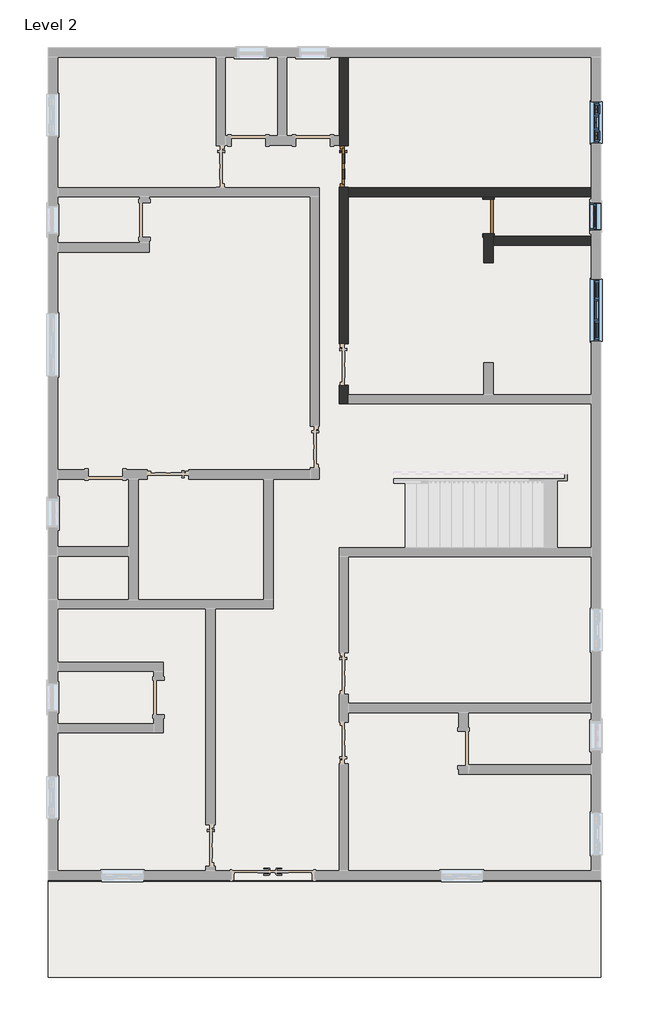
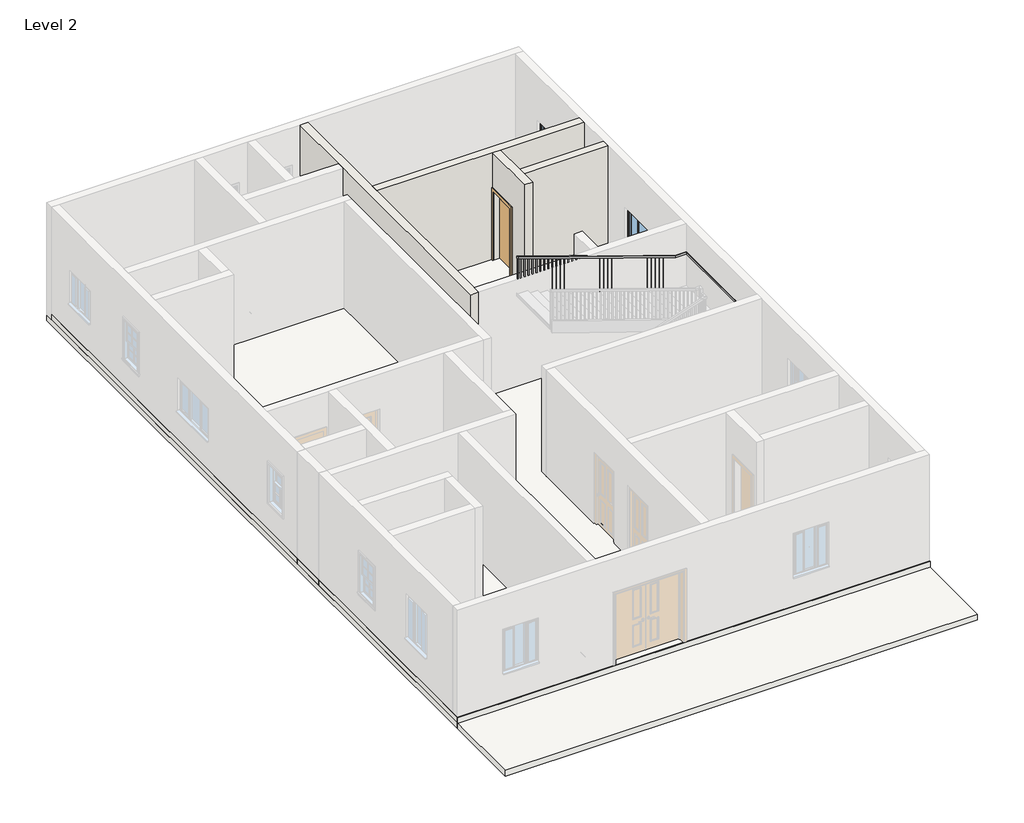
# One storey, part 2 of 3: 4 walls, 3 windows, 2 doors, 2 roofs, 2 slabs, 1 railing.
"""IFC4 building model written with IfcOpenShell, lengths in millimetres."""

from ifc_helpers import new_model, si_unit, frame, origin, place, context, project, spatial, polyline, outline, extrude, faceted_brep, transform, mapped, element, save
from components import door_51b0c682, door_fadea3f2, window_679d2811, windows_tpl_plain_1360x910mm_84993ef1, windows_tpl_w_glazing_cross_bars_910x910mm_4aa0f884

model = new_model("IFC4")

# Units and contexts
model_context = context("Model", 3, world=origin())
ifc_project = project(units=[si_unit("LENGTHUNIT", "METRE", prefix="MILLI")], contexts=[model_context])

# Site, building, storey
site = spatial("IfcSite", under=ifc_project)
building = spatial("IfcBuilding", under=site)
storey = spatial("IfcBuildingStorey", under=building, Name="Level 2", Elevation=3048.0)

# Doors
placement = place(None, origin())
door_shape = door_51b0c682(model_context)
element("IfcDoor", 1, ObjectType="Doors_ExtSgl_2 : 2'x7\"", at=placement, inside=storey, context=model_context, shape_type="MappedRepresentation", body=[
    mapped(door_shape, transform((348.5548051, 6357.8803322, 3048.0), x_axis=(0.0, -1.0, 0.0), y_axis=(1.0, 0.0, 0.0), z_axis=(0.0, 0.0, 1.0))),
])
door_2_shape = door_fadea3f2(model_context)
element("IfcDoor", 2, ObjectType="Single-Flush : 30\" x 80\"", at=placement, inside=storey, context=model_context, shape_type="MappedRepresentation", body=[
    mapped(door_2_shape, transform((3523.5548051, 5259.3303322, 3048.0), x_axis=(0.0, -1.0, 0.0), y_axis=(1.0, 0.0, 0.0), z_axis=(0.0, 0.0, 1.0))),
])

# Railing
element("IfcRailing", 3, ObjectType="Handrail - Rectangular", at=placement, inside=storey, context=model_context, shape_type="SolidModel", body=[
    faceted_brep([(1449.3932247, -2014.4659014, 4048.125), (1449.3932247, -2014.4659014, 3994.4913852), (1449.3932247, -2065.2659014, 3994.4913852), (1449.3932247, -2065.2659014, 4048.125), (5246.6669505, -2014.4659014, 5334.0), (5255.0348019, -2014.4659014, 5283.2), (5255.0348019, -2065.2659014, 5283.2), (5246.6669505, -2065.2659014, 5334.0), (5771.4548051, -2014.4659014, 5334.0), (5771.4548051, -2014.4659014, 5283.2), (5822.2548051, -2065.2659014, 5283.2), (5822.2548051, -2065.2659014, 5334.0), (5771.4548051, 1135.1340986, 5334.0), (5771.4548051, 1135.1340986, 5283.2), (5822.2548051, 1185.9340986, 5283.2), (5822.2548051, 1185.9340986, 5334.0), (5499.8185322, 1135.1340986, 5334.0), (5491.4506807, 1135.1340986, 5283.2), (5491.4506807, 1185.9340986, 5283.2), (5499.8185322, 1185.9340986, 5334.0), (1449.3932247, 1135.1340986, 6705.6), (1449.3932247, 1185.9340986, 6705.6), (1449.3932247, 1185.9340986, 6651.9663852), (1449.3932247, 1135.1340986, 6651.9663852)], [[[0, 1, 2, 3]], [[1, 0, 4, 5]], [[2, 1, 5, 6]], [[3, 2, 6, 7]], [[0, 3, 7, 4]], [[5, 4, 8, 9]], [[6, 5, 9, 10]], [[7, 6, 10, 11]], [[4, 7, 11, 8]], [[9, 8, 12, 13]], [[10, 9, 13, 14]], [[11, 10, 14, 15]], [[8, 11, 15, 12]], [[13, 12, 16, 17]], [[14, 13, 17, 18]], [[15, 14, 18, 19]], [[12, 15, 19, 16]], [[20, 21, 22, 23]], [[17, 16, 20, 23]], [[18, 17, 23, 22]], [[19, 18, 22, 21]], [[16, 19, 21, 20]]]),
    extrude(outline(polyline([(6621.5618562, 1539.1798051), (6628.0127788, 1520.1298051), (5705.475, 1520.1298051), (5705.475, 1539.1798051), (6621.5618562, 1539.1798051)])), frame((0.0, 1151.0090986, 0.0), z_axis=(0.0, 1.0, 0.0), x_axis=(0.0, 0.0, 1.0)), (0.0, 0.0, 1.0), 19.05),
    extrude(outline(polyline([(6587.1569359, 1640.7798051), (6593.6078585, 1621.7298051), (5705.475, 1621.7298051), (5705.475, 1640.7798051), (6587.1569359, 1640.7798051)])), frame((0.0, 1151.0090986, 0.0), z_axis=(0.0, 1.0, 0.0), x_axis=(0.0, 0.0, 1.0)), (0.0, 0.0, 1.0), 19.05),
    extrude(outline(polyline([(6552.7520156, 1742.3798051), (6559.2029381, 1723.3298051), (5619.75, 1723.3298051), (5619.75, 1742.3798051), (6552.7520156, 1742.3798051)])), frame((0.0, 1151.0090986, 0.0), z_axis=(0.0, 1.0, 0.0), x_axis=(0.0, 0.0, 1.0)), (0.0, 0.0, 1.0), 19.05),
    extrude(outline(polyline([(6518.3470953, 1843.9798051), (6524.7980178, 1824.9298051), (5619.75, 1824.9298051), (5619.75, 1843.9798051), (6518.3470953, 1843.9798051)])), frame((0.0, 1151.0090986, 0.0), z_axis=(0.0, 1.0, 0.0), x_axis=(0.0, 0.0, 1.0)), (0.0, 0.0, 1.0), 19.05),
    extrude(outline(polyline([(6483.9421749, 1945.5798051), (6490.3930975, 1926.5298051), (5619.75, 1926.5298051), (5619.75, 1945.5798051), (6483.9421749, 1945.5798051)])), frame((0.0, 1151.0090986, 0.0), z_axis=(0.0, 1.0, 0.0), x_axis=(0.0, 0.0, 1.0)), (0.0, 0.0, 1.0), 19.05),
    extrude(outline(polyline([(6449.5372546, 2047.1798051), (6455.9881772, 2028.1298051), (5534.025, 2028.1298051), (5534.025, 2047.1798051), (6449.5372546, 2047.1798051)])), frame((0.0, 1151.0090986, 0.0), z_axis=(0.0, 1.0, 0.0), x_axis=(0.0, 0.0, 1.0)), (0.0, 0.0, 1.0), 19.05),
    extrude(outline(polyline([(6415.1323343, 2148.7798051), (6421.5832568, 2129.7298051), (5534.025, 2129.7298051), (5534.025, 2148.7798051), (6415.1323343, 2148.7798051)])), frame((0.0, 1151.0090986, 0.0), z_axis=(0.0, 1.0, 0.0), x_axis=(0.0, 0.0, 1.0)), (0.0, 0.0, 1.0), 19.05),
    extrude(outline(polyline([(6380.7274139, 2250.3798051), (6387.1783365, 2231.3298051), (5448.3, 2231.3298051), (5448.3, 2250.3798051), (6380.7274139, 2250.3798051)])), frame((0.0, 1151.0090986, 0.0), z_axis=(0.0, 1.0, 0.0), x_axis=(0.0, 0.0, 1.0)), (0.0, 0.0, 1.0), 19.05),
    extrude(outline(polyline([(6346.3224936, 2351.9798051), (6352.7734162, 2332.9298051), (5448.3, 2332.9298051), (5448.3, 2351.9798051), (6346.3224936, 2351.9798051)])), frame((0.0, 1151.0090986, 0.0), z_axis=(0.0, 1.0, 0.0), x_axis=(0.0, 0.0, 1.0)), (0.0, 0.0, 1.0), 19.05),
    extrude(outline(polyline([(6311.9175733, 2453.5798051), (6318.3684958, 2434.5298051), (5448.3, 2434.5298051), (5448.3, 2453.5798051), (6311.9175733, 2453.5798051)])), frame((0.0, 1151.0090986, 0.0), z_axis=(0.0, 1.0, 0.0), x_axis=(0.0, 0.0, 1.0)), (0.0, 0.0, 1.0), 19.05),
    extrude(outline(polyline([(6277.512653, 2555.1798051), (6283.9635755, 2536.1298051), (5362.575, 2536.1298051), (5362.575, 2555.1798051), (6277.512653, 2555.1798051)])), frame((0.0, 1151.0090986, 0.0), z_axis=(0.0, 1.0, 0.0), x_axis=(0.0, 0.0, 1.0)), (0.0, 0.0, 1.0), 19.05),
    extrude(outline(polyline([(6243.1077326, 2656.7798051), (6249.5586552, 2637.7298051), (5362.575, 2637.7298051), (5362.575, 2656.7798051), (6243.1077326, 2656.7798051)])), frame((0.0, 1151.0090986, 0.0), z_axis=(0.0, 1.0, 0.0), x_axis=(0.0, 0.0, 1.0)), (0.0, 0.0, 1.0), 19.05),
    extrude(outline(polyline([(6208.7028123, 2758.3798051), (6215.1537349, 2739.3298051), (5276.85, 2739.3298051), (5276.85, 2758.3798051), (6208.7028123, 2758.3798051)])), frame((0.0, 1151.0090986, 0.0), z_axis=(0.0, 1.0, 0.0), x_axis=(0.0, 0.0, 1.0)), (0.0, 0.0, 1.0), 19.05),
    extrude(outline(polyline([(6174.297892, 2859.9798051), (6180.7488145, 2840.9298051), (5276.85, 2840.9298051), (5276.85, 2859.9798051), (6174.297892, 2859.9798051)])), frame((0.0, 1151.0090986, 0.0), z_axis=(0.0, 1.0, 0.0), x_axis=(0.0, 0.0, 1.0)), (0.0, 0.0, 1.0), 19.05),
    extrude(outline(polyline([(6139.8929716, 2961.5798051), (6146.3438942, 2942.5298051), (5276.85, 2942.5298051), (5276.85, 2961.5798051), (6139.8929716, 2961.5798051)])), frame((0.0, 1151.0090986, 0.0), z_axis=(0.0, 1.0, 0.0), x_axis=(0.0, 0.0, 1.0)), (0.0, 0.0, 1.0), 19.05),
    extrude(outline(polyline([(6105.4880513, 3063.1798051), (6111.9389739, 3044.1298051), (5191.125, 3044.1298051), (5191.125, 3063.1798051), (6105.4880513, 3063.1798051)])), frame((0.0, 1151.0090986, 0.0), z_axis=(0.0, 1.0, 0.0), x_axis=(0.0, 0.0, 1.0)), (0.0, 0.0, 1.0), 19.05),
    extrude(outline(polyline([(6071.083131, 3164.7798051), (6077.5340535, 3145.7298051), (5191.125, 3145.7298051), (5191.125, 3164.7798051), (6071.083131, 3164.7798051)])), frame((0.0, 1151.0090986, 0.0), z_axis=(0.0, 1.0, 0.0), x_axis=(0.0, 0.0, 1.0)), (0.0, 0.0, 1.0), 19.05),
    extrude(outline(polyline([(6036.6782106, 3266.3798051), (6043.1291332, 3247.3298051), (5105.4, 3247.3298051), (5105.4, 3266.3798051), (6036.6782106, 3266.3798051)])), frame((0.0, 1151.0090986, 0.0), z_axis=(0.0, 1.0, 0.0), x_axis=(0.0, 0.0, 1.0)), (0.0, 0.0, 1.0), 19.05),
    extrude(outline(polyline([(6002.2732903, 3367.9798051), (6008.7242129, 3348.9298051), (5105.4, 3348.9298051), (5105.4, 3367.9798051), (6002.2732903, 3367.9798051)])), frame((0.0, 1151.0090986, 0.0), z_axis=(0.0, 1.0, 0.0), x_axis=(0.0, 0.0, 1.0)), (0.0, 0.0, 1.0), 19.05),
    extrude(outline(polyline([(5967.86837, 3469.5798051), (5974.3192926, 3450.5298051), (5105.4, 3450.5298051), (5105.4, 3469.5798051), (5967.86837, 3469.5798051)])), frame((0.0, 1151.0090986, 0.0), z_axis=(0.0, 1.0, 0.0), x_axis=(0.0, 0.0, 1.0)), (0.0, 0.0, 1.0), 19.05),
    extrude(outline(polyline([(5933.4634497, 3571.1798051), (5939.9143722, 3552.1298051), (5019.675, 3552.1298051), (5019.675, 3571.1798051), (5933.4634497, 3571.1798051)])), frame((0.0, 1151.0090986, 0.0), z_axis=(0.0, 1.0, 0.0), x_axis=(0.0, 0.0, 1.0)), (0.0, 0.0, 1.0), 19.05),
    extrude(outline(polyline([(5899.0585293, 3672.7798051), (5905.5094519, 3653.7298051), (5019.675, 3653.7298051), (5019.675, 3672.7798051), (5899.0585293, 3672.7798051)])), frame((0.0, 1151.0090986, 0.0), z_axis=(0.0, 1.0, 0.0), x_axis=(0.0, 0.0, 1.0)), (0.0, 0.0, 1.0), 19.05),
    extrude(outline(polyline([(5864.653609, 3774.3798051), (5871.1045316, 3755.3298051), (4933.95, 3755.3298051), (4933.95, 3774.3798051), (5864.653609, 3774.3798051)])), frame((0.0, 1151.0090986, 0.0), z_axis=(0.0, 1.0, 0.0), x_axis=(0.0, 0.0, 1.0)), (0.0, 0.0, 1.0), 19.05),
    extrude(outline(polyline([(5830.2486887, 3875.9798051), (5836.6996112, 3856.9298051), (4933.95, 3856.9298051), (4933.95, 3875.9798051), (5830.2486887, 3875.9798051)])), frame((0.0, 1151.0090986, 0.0), z_axis=(0.0, 1.0, 0.0), x_axis=(0.0, 0.0, 1.0)), (0.0, 0.0, 1.0), 19.05),
    extrude(outline(polyline([(5795.8437683, 3977.5798051), (5802.2946909, 3958.5298051), (4933.95, 3958.5298051), (4933.95, 3977.5798051), (5795.8437683, 3977.5798051)])), frame((0.0, 1151.0090986, 0.0), z_axis=(0.0, 1.0, 0.0), x_axis=(0.0, 0.0, 1.0)), (0.0, 0.0, 1.0), 19.05),
    extrude(outline(polyline([(5761.438848, 4079.1798051), (5767.8897706, 4060.1298051), (4848.225, 4060.1298051), (4848.225, 4079.1798051), (5761.438848, 4079.1798051)])), frame((0.0, 1151.0090986, 0.0), z_axis=(0.0, 1.0, 0.0), x_axis=(0.0, 0.0, 1.0)), (0.0, 0.0, 1.0), 19.05),
    extrude(outline(polyline([(5727.0339277, 4180.7798051), (5733.4848502, 4161.7298051), (4848.225, 4161.7298051), (4848.225, 4180.7798051), (5727.0339277, 4180.7798051)])), frame((0.0, 1151.0090986, 0.0), z_axis=(0.0, 1.0, 0.0), x_axis=(0.0, 0.0, 1.0)), (0.0, 0.0, 1.0), 19.05),
    extrude(outline(polyline([(5692.6290074, 4282.3798051), (5699.0799299, 4263.3298051), (4762.5, 4263.3298051), (4762.5, 4282.3798051), (5692.6290074, 4282.3798051)])), frame((0.0, 1151.0090986, 0.0), z_axis=(0.0, 1.0, 0.0), x_axis=(0.0, 0.0, 1.0)), (0.0, 0.0, 1.0), 19.05),
    extrude(outline(polyline([(5658.224087, 4383.9798051), (5664.6750096, 4364.9298051), (4762.5, 4364.9298051), (4762.5, 4383.9798051), (5658.224087, 4383.9798051)])), frame((0.0, 1151.0090986, 0.0), z_axis=(0.0, 1.0, 0.0), x_axis=(0.0, 0.0, 1.0)), (0.0, 0.0, 1.0), 19.05),
    extrude(outline(polyline([(5623.8191667, 4485.5798051), (5630.2700893, 4466.5298051), (4762.5, 4466.5298051), (4762.5, 4485.5798051), (5623.8191667, 4485.5798051)])), frame((0.0, 1151.0090986, 0.0), z_axis=(0.0, 1.0, 0.0), x_axis=(0.0, 0.0, 1.0)), (0.0, 0.0, 1.0), 19.05),
    extrude(outline(polyline([(5589.4142464, 4587.1798051), (5595.8651689, 4568.1298051), (4676.775, 4568.1298051), (4676.775, 4587.1798051), (5589.4142464, 4587.1798051)])), frame((0.0, 1151.0090986, 0.0), z_axis=(0.0, 1.0, 0.0), x_axis=(0.0, 0.0, 1.0)), (0.0, 0.0, 1.0), 19.05),
    extrude(outline(polyline([(5555.009326, 4688.7798051), (5561.4602486, 4669.7298051), (4676.775, 4669.7298051), (4676.775, 4688.7798051), (5555.009326, 4688.7798051)])), frame((0.0, 1151.0090986, 0.0), z_axis=(0.0, 1.0, 0.0), x_axis=(0.0, 0.0, 1.0)), (0.0, 0.0, 1.0), 19.05),
    extrude(outline(polyline([(5520.6044057, 4790.3798051), (5527.0553283, 4771.3298051), (4591.05, 4771.3298051), (4591.05, 4790.3798051), (5520.6044057, 4790.3798051)])), frame((0.0, 1151.0090986, 0.0), z_axis=(0.0, 1.0, 0.0), x_axis=(0.0, 0.0, 1.0)), (0.0, 0.0, 1.0), 19.05),
    extrude(outline(polyline([(5486.1994854, 4891.9798051), (5492.6504079, 4872.9298051), (4591.05, 4872.9298051), (4591.05, 4891.9798051), (5486.1994854, 4891.9798051)])), frame((0.0, 1151.0090986, 0.0), z_axis=(0.0, 1.0, 0.0), x_axis=(0.0, 0.0, 1.0)), (0.0, 0.0, 1.0), 19.05),
    extrude(outline(polyline([(5451.8163852, 4993.5798051), (5458.2673078, 4974.5298051), (4591.05, 4974.5298051), (4591.05, 4993.5798051), (5451.8163852, 4993.5798051)])), frame((0.0, 1151.0090986, 0.0), z_axis=(0.0, 1.0, 0.0), x_axis=(0.0, 0.0, 1.0)), (0.0, 0.0, 1.0), 19.05),
    extrude(outline(polyline([(5417.3896447, 5095.1798051), (5423.8405673, 5076.1298051), (4505.325, 5076.1298051), (4505.325, 5095.1798051), (5417.3896447, 5095.1798051)])), frame((0.0, 1151.0090986, 0.0), z_axis=(0.0, 1.0, 0.0), x_axis=(0.0, 0.0, 1.0)), (0.0, 0.0, 1.0), 19.05),
    extrude(outline(polyline([(5382.9847244, 5196.7798051), (5389.435647, 5177.7298051), (4505.325, 5177.7298051), (4505.325, 5196.7798051), (5382.9847244, 5196.7798051)])), frame((0.0, 1151.0090986, 0.0), z_axis=(0.0, 1.0, 0.0), x_axis=(0.0, 0.0, 1.0)), (0.0, 0.0, 1.0), 19.05),
    extrude(outline(polyline([(5348.5798041, 5298.3798051), (5355.0307266, 5279.3298051), (4419.6, 5279.3298051), (4419.6, 5298.3798051), (5348.5798041, 5298.3798051)])), frame((0.0, 1151.0090986, 0.0), z_axis=(0.0, 1.0, 0.0), x_axis=(0.0, 0.0, 1.0)), (0.0, 0.0, 1.0), 19.05),
    extrude(outline(polyline([(5314.1748837, 5399.9798051), (5320.6258063, 5380.9298051), (4419.6, 5380.9298051), (4419.6, 5399.9798051), (5314.1748837, 5399.9798051)])), frame((0.0, 1151.0090986, 0.0), z_axis=(0.0, 1.0, 0.0), x_axis=(0.0, 0.0, 1.0)), (0.0, 0.0, 1.0), 19.05),
    extrude(outline(polyline([(5279.7699634, 5501.5798051), (5286.220886, 5482.5298051), (4419.6, 5482.5298051), (4419.6, 5501.5798051), (5279.7699634, 5501.5798051)])), frame((0.0, 1151.0090986, 0.0), z_axis=(0.0, 1.0, 0.0), x_axis=(0.0, 0.0, 1.0)), (0.0, 0.0, 1.0), 19.05),
    extrude(outline(polyline([(5603.1798051, 1170.0590986), (5603.1798051, 1151.0090986), (5584.1298051, 1151.0090986), (5584.1298051, 1170.0590986), (5603.1798051, 1170.0590986)])), frame((0.0, 0.0, 4419.6), z_axis=(0.0, 0.0, 1.0), x_axis=(1.0, 0.0, 0.0)), (0.0, 0.0, 1.0), 863.6),
    extrude(outline(polyline([(5704.7798051, 1170.0590986), (5704.7798051, 1151.0090986), (5685.7298051, 1151.0090986), (5685.7298051, 1170.0590986), (5704.7798051, 1170.0590986)])), frame((0.0, 0.0, 4419.6), z_axis=(0.0, 0.0, 1.0), x_axis=(1.0, 0.0, 0.0)), (0.0, 0.0, 1.0), 863.6),
    extrude(outline(polyline([(5806.3798051, 1100.2090986), (5787.3298051, 1100.2090986), (5787.3298051, 1119.2590986), (5806.3798051, 1119.2590986), (5806.3798051, 1100.2090986)])), frame((0.0, 0.0, 4419.6), z_axis=(0.0, 0.0, 1.0), x_axis=(1.0, 0.0, 0.0)), (0.0, 0.0, 1.0), 863.6),
    extrude(outline(polyline([(5806.3798051, 998.6090986), (5787.3298051, 998.6090986), (5787.3298051, 1017.6590986), (5806.3798051, 1017.6590986), (5806.3798051, 998.6090986)])), frame((0.0, 0.0, 4419.6), z_axis=(0.0, 0.0, 1.0), x_axis=(1.0, 0.0, 0.0)), (0.0, 0.0, 1.0), 863.6),
    extrude(outline(polyline([(5806.3798051, 897.0090986), (5787.3298051, 897.0090986), (5787.3298051, 916.0590986), (5806.3798051, 916.0590986), (5806.3798051, 897.0090986)])), frame((0.0, 0.0, 4419.6), z_axis=(0.0, 0.0, 1.0), x_axis=(1.0, 0.0, 0.0)), (0.0, 0.0, 1.0), 863.6),
    extrude(outline(polyline([(5806.3798051, 795.4090986), (5787.3298051, 795.4090986), (5787.3298051, 814.4590986), (5806.3798051, 814.4590986), (5806.3798051, 795.4090986)])), frame((0.0, 0.0, 4419.6), z_axis=(0.0, 0.0, 1.0), x_axis=(1.0, 0.0, 0.0)), (0.0, 0.0, 1.0), 863.6),
    extrude(outline(polyline([(5806.3798051, 693.8090986), (5787.3298051, 693.8090986), (5787.3298051, 712.8590986), (5806.3798051, 712.8590986), (5806.3798051, 693.8090986)])), frame((0.0, 0.0, 4419.6), z_axis=(0.0, 0.0, 1.0), x_axis=(1.0, 0.0, 0.0)), (0.0, 0.0, 1.0), 863.6),
    extrude(outline(polyline([(5806.3798051, 592.2090986), (5787.3298051, 592.2090986), (5787.3298051, 611.2590986), (5806.3798051, 611.2590986), (5806.3798051, 592.2090986)])), frame((0.0, 0.0, 4419.6), z_axis=(0.0, 0.0, 1.0), x_axis=(1.0, 0.0, 0.0)), (0.0, 0.0, 1.0), 863.6),
    extrude(outline(polyline([(5806.3798051, 490.6090986), (5787.3298051, 490.6090986), (5787.3298051, 509.6590986), (5806.3798051, 509.6590986), (5806.3798051, 490.6090986)])), frame((0.0, 0.0, 4419.6), z_axis=(0.0, 0.0, 1.0), x_axis=(1.0, 0.0, 0.0)), (0.0, 0.0, 1.0), 863.6),
    extrude(outline(polyline([(5806.3798051, 389.0090986), (5787.3298051, 389.0090986), (5787.3298051, 408.0590986), (5806.3798051, 408.0590986), (5806.3798051, 389.0090986)])), frame((0.0, 0.0, 4419.6), z_axis=(0.0, 0.0, 1.0), x_axis=(1.0, 0.0, 0.0)), (0.0, 0.0, 1.0), 863.6),
    extrude(outline(polyline([(5806.3798051, 287.4090986), (5787.3298051, 287.4090986), (5787.3298051, 306.4590986), (5806.3798051, 306.4590986), (5806.3798051, 287.4090986)])), frame((0.0, 0.0, 4419.6), z_axis=(0.0, 0.0, 1.0), x_axis=(1.0, 0.0, 0.0)), (0.0, 0.0, 1.0), 863.6),
    extrude(outline(polyline([(5806.3798051, 185.8090986), (5787.3298051, 185.8090986), (5787.3298051, 204.8590986), (5806.3798051, 204.8590986), (5806.3798051, 185.8090986)])), frame((0.0, 0.0, 4419.6), z_axis=(0.0, 0.0, 1.0), x_axis=(1.0, 0.0, 0.0)), (0.0, 0.0, 1.0), 863.6),
    extrude(outline(polyline([(5806.3798051, 84.2090986), (5787.3298051, 84.2090986), (5787.3298051, 103.2590986), (5806.3798051, 103.2590986), (5806.3798051, 84.2090986)])), frame((0.0, 0.0, 4419.6), z_axis=(0.0, 0.0, 1.0), x_axis=(1.0, 0.0, 0.0)), (0.0, 0.0, 1.0), 863.6),
    extrude(outline(polyline([(5806.3798051, -17.3909014), (5787.3298051, -17.3909014), (5787.3298051, 1.6590986), (5806.3798051, 1.6590986), (5806.3798051, -17.3909014)])), frame((0.0, 0.0, 4419.6), z_axis=(0.0, 0.0, 1.0), x_axis=(1.0, 0.0, 0.0)), (0.0, 0.0, 1.0), 863.6),
    extrude(outline(polyline([(5806.3798051, -118.9909014), (5787.3298051, -118.9909014), (5787.3298051, -99.9409014), (5806.3798051, -99.9409014), (5806.3798051, -118.9909014)])), frame((0.0, 0.0, 4419.6), z_axis=(0.0, 0.0, 1.0), x_axis=(1.0, 0.0, 0.0)), (0.0, 0.0, 1.0), 863.6),
    extrude(outline(polyline([(5806.3798051, -220.5909014), (5787.3298051, -220.5909014), (5787.3298051, -201.5409014), (5806.3798051, -201.5409014), (5806.3798051, -220.5909014)])), frame((0.0, 0.0, 4419.6), z_axis=(0.0, 0.0, 1.0), x_axis=(1.0, 0.0, 0.0)), (0.0, 0.0, 1.0), 863.6),
    extrude(outline(polyline([(5806.3798051, -322.1909014), (5787.3298051, -322.1909014), (5787.3298051, -303.1409014), (5806.3798051, -303.1409014), (5806.3798051, -322.1909014)])), frame((0.0, 0.0, 4419.6), z_axis=(0.0, 0.0, 1.0), x_axis=(1.0, 0.0, 0.0)), (0.0, 0.0, 1.0), 863.6),
    extrude(outline(polyline([(5806.3798051, -423.7909014), (5787.3298051, -423.7909014), (5787.3298051, -404.7409014), (5806.3798051, -404.7409014), (5806.3798051, -423.7909014)])), frame((0.0, 0.0, 4419.6), z_axis=(0.0, 0.0, 1.0), x_axis=(1.0, 0.0, 0.0)), (0.0, 0.0, 1.0), 863.6),
    extrude(outline(polyline([(5806.3798051, -525.3909014), (5787.3298051, -525.3909014), (5787.3298051, -506.3409014), (5806.3798051, -506.3409014), (5806.3798051, -525.3909014)])), frame((0.0, 0.0, 4419.6), z_axis=(0.0, 0.0, 1.0), x_axis=(1.0, 0.0, 0.0)), (0.0, 0.0, 1.0), 863.6),
    extrude(outline(polyline([(5806.3798051, -626.9909014), (5787.3298051, -626.9909014), (5787.3298051, -607.9409014), (5806.3798051, -607.9409014), (5806.3798051, -626.9909014)])), frame((0.0, 0.0, 4419.6), z_axis=(0.0, 0.0, 1.0), x_axis=(1.0, 0.0, 0.0)), (0.0, 0.0, 1.0), 863.6),
    extrude(outline(polyline([(5806.3798051, -728.5909014), (5787.3298051, -728.5909014), (5787.3298051, -709.5409014), (5806.3798051, -709.5409014), (5806.3798051, -728.5909014)])), frame((0.0, 0.0, 4419.6), z_axis=(0.0, 0.0, 1.0), x_axis=(1.0, 0.0, 0.0)), (0.0, 0.0, 1.0), 863.6),
    extrude(outline(polyline([(5806.3798051, -830.1909014), (5787.3298051, -830.1909014), (5787.3298051, -811.1409014), (5806.3798051, -811.1409014), (5806.3798051, -830.1909014)])), frame((0.0, 0.0, 4419.6), z_axis=(0.0, 0.0, 1.0), x_axis=(1.0, 0.0, 0.0)), (0.0, 0.0, 1.0), 863.6),
    extrude(outline(polyline([(5806.3798051, -931.7909014), (5787.3298051, -931.7909014), (5787.3298051, -912.7409014), (5806.3798051, -912.7409014), (5806.3798051, -931.7909014)])), frame((0.0, 0.0, 4419.6), z_axis=(0.0, 0.0, 1.0), x_axis=(1.0, 0.0, 0.0)), (0.0, 0.0, 1.0), 863.6),
    extrude(outline(polyline([(5806.3798051, -1033.3909014), (5787.3298051, -1033.3909014), (5787.3298051, -1014.3409014), (5806.3798051, -1014.3409014), (5806.3798051, -1033.3909014)])), frame((0.0, 0.0, 4419.6), z_axis=(0.0, 0.0, 1.0), x_axis=(1.0, 0.0, 0.0)), (0.0, 0.0, 1.0), 863.6),
    extrude(outline(polyline([(5806.3798051, -1134.9909014), (5787.3298051, -1134.9909014), (5787.3298051, -1115.9409014), (5806.3798051, -1115.9409014), (5806.3798051, -1134.9909014)])), frame((0.0, 0.0, 4419.6), z_axis=(0.0, 0.0, 1.0), x_axis=(1.0, 0.0, 0.0)), (0.0, 0.0, 1.0), 863.6),
    extrude(outline(polyline([(5806.3798051, -1236.5909014), (5787.3298051, -1236.5909014), (5787.3298051, -1217.5409014), (5806.3798051, -1217.5409014), (5806.3798051, -1236.5909014)])), frame((0.0, 0.0, 4419.6), z_axis=(0.0, 0.0, 1.0), x_axis=(1.0, 0.0, 0.0)), (0.0, 0.0, 1.0), 863.6),
    extrude(outline(polyline([(5806.3798051, -1338.1909014), (5787.3298051, -1338.1909014), (5787.3298051, -1319.1409014), (5806.3798051, -1319.1409014), (5806.3798051, -1338.1909014)])), frame((0.0, 0.0, 4419.6), z_axis=(0.0, 0.0, 1.0), x_axis=(1.0, 0.0, 0.0)), (0.0, 0.0, 1.0), 863.6),
    extrude(outline(polyline([(5806.3798051, -1439.7909014), (5787.3298051, -1439.7909014), (5787.3298051, -1420.7409014), (5806.3798051, -1420.7409014), (5806.3798051, -1439.7909014)])), frame((0.0, 0.0, 4419.6), z_axis=(0.0, 0.0, 1.0), x_axis=(1.0, 0.0, 0.0)), (0.0, 0.0, 1.0), 863.6),
    extrude(outline(polyline([(5806.3798051, -1541.3909014), (5787.3298051, -1541.3909014), (5787.3298051, -1522.3409014), (5806.3798051, -1522.3409014), (5806.3798051, -1541.3909014)])), frame((0.0, 0.0, 4419.6), z_axis=(0.0, 0.0, 1.0), x_axis=(1.0, 0.0, 0.0)), (0.0, 0.0, 1.0), 863.6),
    extrude(outline(polyline([(5806.3798051, -1642.9909014), (5787.3298051, -1642.9909014), (5787.3298051, -1623.9409014), (5806.3798051, -1623.9409014), (5806.3798051, -1642.9909014)])), frame((0.0, 0.0, 4419.6), z_axis=(0.0, 0.0, 1.0), x_axis=(1.0, 0.0, 0.0)), (0.0, 0.0, 1.0), 863.6),
    extrude(outline(polyline([(5806.3798051, -1744.5909014), (5787.3298051, -1744.5909014), (5787.3298051, -1725.5409014), (5806.3798051, -1725.5409014), (5806.3798051, -1744.5909014)])), frame((0.0, 0.0, 4419.6), z_axis=(0.0, 0.0, 1.0), x_axis=(1.0, 0.0, 0.0)), (0.0, 0.0, 1.0), 863.6),
    extrude(outline(polyline([(5806.3798051, -1846.1909014), (5787.3298051, -1846.1909014), (5787.3298051, -1827.1409014), (5806.3798051, -1827.1409014), (5806.3798051, -1846.1909014)])), frame((0.0, 0.0, 4419.6), z_axis=(0.0, 0.0, 1.0), x_axis=(1.0, 0.0, 0.0)), (0.0, 0.0, 1.0), 863.6),
    extrude(outline(polyline([(5806.3798051, -1947.7909014), (5787.3298051, -1947.7909014), (5787.3298051, -1928.7409014), (5806.3798051, -1928.7409014), (5806.3798051, -1947.7909014)])), frame((0.0, 0.0, 4419.6), z_axis=(0.0, 0.0, 1.0), x_axis=(1.0, 0.0, 0.0)), (0.0, 0.0, 1.0), 863.6),
    extrude(outline(polyline([(5707.0682247, -2049.3909014), (5707.0682247, -2030.3409014), (5726.1182247, -2030.3409014), (5726.1182247, -2049.3909014), (5707.0682247, -2049.3909014)])), frame((0.0, 0.0, 4419.6), z_axis=(0.0, 0.0, 1.0), x_axis=(1.0, 0.0, 0.0)), (0.0, 0.0, 1.0), 863.6),
    extrude(outline(polyline([(5605.4682247, -2049.3909014), (5605.4682247, -2030.3409014), (5624.5182247, -2030.3409014), (5624.5182247, -2049.3909014), (5605.4682247, -2049.3909014)])), frame((0.0, 0.0, 4419.6), z_axis=(0.0, 0.0, 1.0), x_axis=(1.0, 0.0, 0.0)), (0.0, 0.0, 1.0), 863.6),
    extrude(outline(polyline([(5503.8682247, -2049.3909014), (5503.8682247, -2030.3409014), (5522.9182247, -2030.3409014), (5522.9182247, -2049.3909014), (5503.8682247, -2049.3909014)])), frame((0.0, 0.0, 4419.6), z_axis=(0.0, 0.0, 1.0), x_axis=(1.0, 0.0, 0.0)), (0.0, 0.0, 1.0), 863.6),
    extrude(outline(polyline([(5402.2682247, -2049.3909014), (5402.2682247, -2030.3409014), (5421.3182247, -2030.3409014), (5421.3182247, -2049.3909014), (5402.2682247, -2049.3909014)])), frame((0.0, 0.0, 4419.6), z_axis=(0.0, 0.0, 1.0), x_axis=(1.0, 0.0, 0.0)), (0.0, 0.0, 1.0), 863.6),
    extrude(outline(polyline([(5300.6682247, -2049.3909014), (5300.6682247, -2030.3409014), (5319.7182247, -2030.3409014), (5319.7182247, -2049.3909014), (5300.6682247, -2049.3909014)])), frame((0.0, 0.0, 4419.6), z_axis=(0.0, 0.0, 1.0), x_axis=(1.0, 0.0, 0.0)), (0.0, 0.0, 1.0), 863.6),
    extrude(outline(polyline([(5270.6988987, 5218.1182247), (5264.2479761, 5199.0682247), (4333.875, 5199.0682247), (4333.875, 5218.1182247), (5270.6988987, 5218.1182247)])), frame((0.0, -2049.3909014, 0.0), z_axis=(0.0, 1.0, 0.0), x_axis=(0.0, 0.0, 1.0)), (0.0, 0.0, 1.0), 19.05),
    extrude(outline(polyline([(5236.2939783, 5116.5182247), (5229.8430558, 5097.4682247), (4333.875, 5097.4682247), (4333.875, 5116.5182247), (5236.2939783, 5116.5182247)])), frame((0.0, -2049.3909014, 0.0), z_axis=(0.0, 1.0, 0.0), x_axis=(0.0, 0.0, 1.0)), (0.0, 0.0, 1.0), 19.05),
    extrude(outline(polyline([(5201.889058, 5014.9182247), (5195.4381354, 4995.8682247), (4333.875, 4995.8682247), (4333.875, 5014.9182247), (5201.889058, 5014.9182247)])), frame((0.0, -2049.3909014, 0.0), z_axis=(0.0, 1.0, 0.0), x_axis=(0.0, 0.0, 1.0)), (0.0, 0.0, 1.0), 19.05),
    extrude(outline(polyline([(5167.4841377, 4913.3182247), (5161.0332151, 4894.2682247), (4248.15, 4894.2682247), (4248.15, 4913.3182247), (5167.4841377, 4913.3182247)])), frame((0.0, -2049.3909014, 0.0), z_axis=(0.0, 1.0, 0.0), x_axis=(0.0, 0.0, 1.0)), (0.0, 0.0, 1.0), 19.05),
    extrude(outline(polyline([(5133.0792173, 4811.7182247), (5126.6282948, 4792.6682247), (4248.15, 4792.6682247), (4248.15, 4811.7182247), (5133.0792173, 4811.7182247)])), frame((0.0, -2049.3909014, 0.0), z_axis=(0.0, 1.0, 0.0), x_axis=(0.0, 0.0, 1.0)), (0.0, 0.0, 1.0), 19.05),
    extrude(outline(polyline([(5098.674297, 4710.1182247), (5092.2233745, 4691.0682247), (4162.425, 4691.0682247), (4162.425, 4710.1182247), (5098.674297, 4710.1182247)])), frame((0.0, -2049.3909014, 0.0), z_axis=(0.0, 1.0, 0.0), x_axis=(0.0, 0.0, 1.0)), (0.0, 0.0, 1.0), 19.05),
    extrude(outline(polyline([(5064.2693767, 4608.5182247), (5057.8184541, 4589.4682247), (4162.425, 4589.4682247), (4162.425, 4608.5182247), (5064.2693767, 4608.5182247)])), frame((0.0, -2049.3909014, 0.0), z_axis=(0.0, 1.0, 0.0), x_axis=(0.0, 0.0, 1.0)), (0.0, 0.0, 1.0), 19.05),
    extrude(outline(polyline([(5029.8644564, 4506.9182247), (5023.4135338, 4487.8682247), (4162.425, 4487.8682247), (4162.425, 4506.9182247), (5029.8644564, 4506.9182247)])), frame((0.0, -2049.3909014, 0.0), z_axis=(0.0, 1.0, 0.0), x_axis=(0.0, 0.0, 1.0)), (0.0, 0.0, 1.0), 19.05),
    extrude(outline(polyline([(4995.459536, 4405.3182247), (4989.0086135, 4386.2682247), (4076.7, 4386.2682247), (4076.7, 4405.3182247), (4995.459536, 4405.3182247)])), frame((0.0, -2049.3909014, 0.0), z_axis=(0.0, 1.0, 0.0), x_axis=(0.0, 0.0, 1.0)), (0.0, 0.0, 1.0), 19.05),
    extrude(outline(polyline([(4961.0546157, 4303.7182247), (4954.6036931, 4284.6682247), (4076.7, 4284.6682247), (4076.7, 4303.7182247), (4961.0546157, 4303.7182247)])), frame((0.0, -2049.3909014, 0.0), z_axis=(0.0, 1.0, 0.0), x_axis=(0.0, 0.0, 1.0)), (0.0, 0.0, 1.0), 19.05),
    extrude(outline(polyline([(4926.6496954, 4202.1182247), (4920.1987728, 4183.0682247), (3990.975, 4183.0682247), (3990.975, 4202.1182247), (4926.6496954, 4202.1182247)])), frame((0.0, -2049.3909014, 0.0), z_axis=(0.0, 1.0, 0.0), x_axis=(0.0, 0.0, 1.0)), (0.0, 0.0, 1.0), 19.05),
    extrude(outline(polyline([(4892.244775, 4100.5182247), (4885.7938525, 4081.4682247), (3990.975, 4081.4682247), (3990.975, 4100.5182247), (4892.244775, 4100.5182247)])), frame((0.0, -2049.3909014, 0.0), z_axis=(0.0, 1.0, 0.0), x_axis=(0.0, 0.0, 1.0)), (0.0, 0.0, 1.0), 19.05),
    extrude(outline(polyline([(4857.8398547, 3998.9182247), (4851.3889321, 3979.8682247), (3990.975, 3979.8682247), (3990.975, 3998.9182247), (4857.8398547, 3998.9182247)])), frame((0.0, -2049.3909014, 0.0), z_axis=(0.0, 1.0, 0.0), x_axis=(0.0, 0.0, 1.0)), (0.0, 0.0, 1.0), 19.05),
    extrude(outline(polyline([(4823.4349344, 3897.3182247), (4816.9840118, 3878.2682247), (3905.25, 3878.2682247), (3905.25, 3897.3182247), (4823.4349344, 3897.3182247)])), frame((0.0, -2049.3909014, 0.0), z_axis=(0.0, 1.0, 0.0), x_axis=(0.0, 0.0, 1.0)), (0.0, 0.0, 1.0), 19.05),
    extrude(outline(polyline([(4789.0300141, 3795.7182247), (4782.5790915, 3776.6682247), (3905.25, 3776.6682247), (3905.25, 3795.7182247), (4789.0300141, 3795.7182247)])), frame((0.0, -2049.3909014, 0.0), z_axis=(0.0, 1.0, 0.0), x_axis=(0.0, 0.0, 1.0)), (0.0, 0.0, 1.0), 19.05),
    extrude(outline(polyline([(4754.6250937, 3694.1182247), (4748.1741712, 3675.0682247), (3819.525, 3675.0682247), (3819.525, 3694.1182247), (4754.6250937, 3694.1182247)])), frame((0.0, -2049.3909014, 0.0), z_axis=(0.0, 1.0, 0.0), x_axis=(0.0, 0.0, 1.0)), (0.0, 0.0, 1.0), 19.05),
    extrude(outline(polyline([(4720.2201734, 3592.5182247), (4713.7692508, 3573.4682247), (3819.525, 3573.4682247), (3819.525, 3592.5182247), (4720.2201734, 3592.5182247)])), frame((0.0, -2049.3909014, 0.0), z_axis=(0.0, 1.0, 0.0), x_axis=(0.0, 0.0, 1.0)), (0.0, 0.0, 1.0), 19.05),
    extrude(outline(polyline([(4685.8152531, 3490.9182247), (4679.3643305, 3471.8682247), (3819.525, 3471.8682247), (3819.525, 3490.9182247), (4685.8152531, 3490.9182247)])), frame((0.0, -2049.3909014, 0.0), z_axis=(0.0, 1.0, 0.0), x_axis=(0.0, 0.0, 1.0)), (0.0, 0.0, 1.0), 19.05),
    extrude(outline(polyline([(4651.4103327, 3389.3182247), (4644.9594102, 3370.2682247), (3733.8, 3370.2682247), (3733.8, 3389.3182247), (4651.4103327, 3389.3182247)])), frame((0.0, -2049.3909014, 0.0), z_axis=(0.0, 1.0, 0.0), x_axis=(0.0, 0.0, 1.0)), (0.0, 0.0, 1.0), 19.05),
    extrude(outline(polyline([(4617.0054124, 3287.7182247), (4610.5544898, 3268.6682247), (3733.8, 3268.6682247), (3733.8, 3287.7182247), (4617.0054124, 3287.7182247)])), frame((0.0, -2049.3909014, 0.0), z_axis=(0.0, 1.0, 0.0), x_axis=(0.0, 0.0, 1.0)), (0.0, 0.0, 1.0), 19.05),
    extrude(outline(polyline([(4582.6004921, 3186.1182247), (4576.1495695, 3167.0682247), (3648.075, 3167.0682247), (3648.075, 3186.1182247), (4582.6004921, 3186.1182247)])), frame((0.0, -2049.3909014, 0.0), z_axis=(0.0, 1.0, 0.0), x_axis=(0.0, 0.0, 1.0)), (0.0, 0.0, 1.0), 19.05),
    extrude(outline(polyline([(4548.1955718, 3084.5182247), (4541.7446492, 3065.4682247), (3648.075, 3065.4682247), (3648.075, 3084.5182247), (4548.1955718, 3084.5182247)])), frame((0.0, -2049.3909014, 0.0), z_axis=(0.0, 1.0, 0.0), x_axis=(0.0, 0.0, 1.0)), (0.0, 0.0, 1.0), 19.05),
    extrude(outline(polyline([(4513.7906514, 2982.9182247), (4507.3397289, 2963.8682247), (3648.075, 2963.8682247), (3648.075, 2982.9182247), (4513.7906514, 2982.9182247)])), frame((0.0, -2049.3909014, 0.0), z_axis=(0.0, 1.0, 0.0), x_axis=(0.0, 0.0, 1.0)), (0.0, 0.0, 1.0), 19.05),
    extrude(outline(polyline([(4479.3857311, 2881.3182247), (4472.9348085, 2862.2682247), (3562.35, 2862.2682247), (3562.35, 2881.3182247), (4479.3857311, 2881.3182247)])), frame((0.0, -2049.3909014, 0.0), z_axis=(0.0, 1.0, 0.0), x_axis=(0.0, 0.0, 1.0)), (0.0, 0.0, 1.0), 19.05),
    extrude(outline(polyline([(4444.9808108, 2779.7182247), (4438.5298882, 2760.6682247), (3562.35, 2760.6682247), (3562.35, 2779.7182247), (4444.9808108, 2779.7182247)])), frame((0.0, -2049.3909014, 0.0), z_axis=(0.0, 1.0, 0.0), x_axis=(0.0, 0.0, 1.0)), (0.0, 0.0, 1.0), 19.05),
    extrude(outline(polyline([(4410.5758904, 2678.1182247), (4404.1249679, 2659.0682247), (3476.625, 2659.0682247), (3476.625, 2678.1182247), (4410.5758904, 2678.1182247)])), frame((0.0, -2049.3909014, 0.0), z_axis=(0.0, 1.0, 0.0), x_axis=(0.0, 0.0, 1.0)), (0.0, 0.0, 1.0), 19.05),
    extrude(outline(polyline([(4376.1709701, 2576.5182247), (4369.7200475, 2557.4682247), (3476.625, 2557.4682247), (3476.625, 2576.5182247), (4376.1709701, 2576.5182247)])), frame((0.0, -2049.3909014, 0.0), z_axis=(0.0, 1.0, 0.0), x_axis=(0.0, 0.0, 1.0)), (0.0, 0.0, 1.0), 19.05),
    extrude(outline(polyline([(4341.7660498, 2474.9182247), (4335.3151272, 2455.8682247), (3476.625, 2455.8682247), (3476.625, 2474.9182247), (4341.7660498, 2474.9182247)])), frame((0.0, -2049.3909014, 0.0), z_axis=(0.0, 1.0, 0.0), x_axis=(0.0, 0.0, 1.0)), (0.0, 0.0, 1.0), 19.05),
    extrude(outline(polyline([(4307.3611294, 2373.3182247), (4300.9102069, 2354.2682247), (3390.9, 2354.2682247), (3390.9, 2373.3182247), (4307.3611294, 2373.3182247)])), frame((0.0, -2049.3909014, 0.0), z_axis=(0.0, 1.0, 0.0), x_axis=(0.0, 0.0, 1.0)), (0.0, 0.0, 1.0), 19.05),
    extrude(outline(polyline([(4272.9562091, 2271.7182247), (4266.5052866, 2252.6682247), (3390.9, 2252.6682247), (3390.9, 2271.7182247), (4272.9562091, 2271.7182247)])), frame((0.0, -2049.3909014, 0.0), z_axis=(0.0, 1.0, 0.0), x_axis=(0.0, 0.0, 1.0)), (0.0, 0.0, 1.0), 19.05),
    extrude(outline(polyline([(4238.5512888, 2170.1182247), (4232.1003662, 2151.0682247), (3305.175, 2151.0682247), (3305.175, 2170.1182247), (4238.5512888, 2170.1182247)])), frame((0.0, -2049.3909014, 0.0), z_axis=(0.0, 1.0, 0.0), x_axis=(0.0, 0.0, 1.0)), (0.0, 0.0, 1.0), 19.05),
    extrude(outline(polyline([(4204.1463685, 2068.5182247), (4197.6954459, 2049.4682247), (3305.175, 2049.4682247), (3305.175, 2068.5182247), (4204.1463685, 2068.5182247)])), frame((0.0, -2049.3909014, 0.0), z_axis=(0.0, 1.0, 0.0), x_axis=(0.0, 0.0, 1.0)), (0.0, 0.0, 1.0), 19.05),
    extrude(outline(polyline([(4169.7414481, 1966.9182247), (4163.2905256, 1947.8682247), (3305.175, 1947.8682247), (3305.175, 1966.9182247), (4169.7414481, 1966.9182247)])), frame((0.0, -2049.3909014, 0.0), z_axis=(0.0, 1.0, 0.0), x_axis=(0.0, 0.0, 1.0)), (0.0, 0.0, 1.0), 19.05),
    extrude(outline(polyline([(4135.3365278, 1865.3182247), (4128.8856052, 1846.2682247), (3219.45, 1846.2682247), (3219.45, 1865.3182247), (4135.3365278, 1865.3182247)])), frame((0.0, -2049.3909014, 0.0), z_axis=(0.0, 1.0, 0.0), x_axis=(0.0, 0.0, 1.0)), (0.0, 0.0, 1.0), 19.05),
    extrude(outline(polyline([(4100.9316075, 1763.7182247), (4094.4806849, 1744.6682247), (3219.45, 1744.6682247), (3219.45, 1763.7182247), (4100.9316075, 1763.7182247)])), frame((0.0, -2049.3909014, 0.0), z_axis=(0.0, 1.0, 0.0), x_axis=(0.0, 0.0, 1.0)), (0.0, 0.0, 1.0), 19.05),
    extrude(outline(polyline([(4066.5266871, 1662.1182247), (4060.0757646, 1643.0682247), (3133.725, 1643.0682247), (3133.725, 1662.1182247), (4066.5266871, 1662.1182247)])), frame((0.0, -2049.3909014, 0.0), z_axis=(0.0, 1.0, 0.0), x_axis=(0.0, 0.0, 1.0)), (0.0, 0.0, 1.0), 19.05),
    extrude(outline(polyline([(4032.1217668, 1560.5182247), (4025.6708443, 1541.4682247), (3133.725, 1541.4682247), (3133.725, 1560.5182247), (4032.1217668, 1560.5182247)])), frame((0.0, -2049.3909014, 0.0), z_axis=(0.0, 1.0, 0.0), x_axis=(0.0, 0.0, 1.0)), (0.0, 0.0, 1.0), 19.05),
    extrude(outline(polyline([(5806.3798051, 1151.0090986), (5787.3298051, 1151.0090986), (5787.3298051, 1170.0590986), (5806.3798051, 1170.0590986), (5806.3798051, 1151.0090986)])), frame((0.0, 0.0, 4419.6), z_axis=(0.0, 0.0, 1.0), x_axis=(1.0, 0.0, 0.0)), (0.0, 0.0, 1.0), 863.6),
    extrude(outline(polyline([(5787.3298051, -2049.3909014), (5787.3298051, -2030.3409014), (5806.3798051, -2030.3409014), (5806.3798051, -2049.3909014), (5787.3298051, -2049.3909014)])), frame((0.0, 0.0, 4419.6), z_axis=(0.0, 0.0, 1.0), x_axis=(1.0, 0.0, 0.0)), (0.0, 0.0, 1.0), 863.6),
    extrude(outline(polyline([(6645.5154626, 1468.4432247), (6651.9663852, 1449.3932247), (5705.475, 1449.3932247), (5705.475, 1468.4432247), (6645.5154626, 1468.4432247)])), frame((0.0, 1151.0090986, 0.0), z_axis=(0.0, 1.0, 0.0), x_axis=(0.0, 0.0, 1.0)), (0.0, 0.0, 1.0), 19.05),
    extrude(outline(polyline([(4000.9423078, 1468.4432247), (3994.4913852, 1449.3932247), (3133.725, 1449.3932247), (3133.725, 1468.4432247), (4000.9423078, 1468.4432247)])), frame((0.0, -2049.3909014, 0.0), z_axis=(0.0, 1.0, 0.0), x_axis=(0.0, 0.0, 1.0)), (0.0, 0.0, 1.0), 19.05),
])

# Roofs
element("IfcRoof", 4, ObjectType="Generic - 12\"", at=placement, inside=storey, context=model_context, shape_type="SweptSolid", body=[
    extrude(outline(polyline([(-6134.0560205, 8955.7974079), (5981.7439795, 8955.7974079), (5981.7439795, -9298.1734342), (-6134.0560205, -9298.1734342), (-6134.0560205, 8955.7974079)])), frame((0.0, 0.0, 3048.0), z_axis=(0.0, 0.0, 1.0), x_axis=(1.0, 0.0, 0.0)), (0.0, 0.0, 1.0), 152.4),
])
element("IfcRoof", 5, ObjectType="Generic - 12\"", at=placement, inside=storey, context=model_context, shape_type="SweptSolid", body=[
    extrude(outline(polyline([(-6134.0560205, 8955.7974079), (5981.7439795, 8955.7974079), (5981.7439795, -9323.5734342), (-6134.0560205, -9323.5734342), (-6134.0560205, 8955.7974079)])), frame((0.0, 0.0, 3048.0), z_axis=(0.0, 0.0, 1.0), x_axis=(1.0, 0.0, 0.0)), (0.0, 0.0, 1.0), 152.4),
])

# Slabs
element("IfcSlab", 6, ObjectType="Generic - 12\"", at=placement, inside=storey, context=model_context, shape_type="SweptSolid", body=[
    extrude(outline(polyline([(5981.7439795, 8955.7974079), (5981.7439795, -9298.1734342), (-6134.0560205, -9298.1734342), (-6134.0560205, 8955.7974079), (5981.7439795, 8955.7974079)])), frame((0.0, 0.0, 2895.6), z_axis=(0.0, 0.0, 1.0), x_axis=(1.0, 0.0, 0.0)), (0.0, 0.0, 1.0), 152.4),
])
element("IfcSlab", 7, ObjectType="Generic - 12\"", at=placement, inside=storey, context=model_context, shape_type="SweptSolid", body=[
    extrude(outline(polyline([(5981.7439795, -9298.1734342), (5981.7439795, -11431.7734342), (-6134.0560205, -11431.7734342), (-6134.0560205, -9298.1734342), (5981.7439795, -9298.1734342)])), frame((0.0, 0.0, 2895.6), z_axis=(0.0, 0.0, 1.0), x_axis=(1.0, 0.0, 0.0)), (0.0, 0.0, 1.0), 152.4),
])

# Walls
element("IfcWall", 8, ObjectType="Generic - 4.5\" p", at=placement, inside=storey, context=model_context, shape_type="Brep", body=[
    faceted_brep([(246.9548051, 1556.4340986, 5158.0), (246.9548051, 1556.4340986, 3048.0), (246.9548051, 1147.8340986, 3048.0), (246.9548051, 1147.8340986, 6096.0), (246.9548051, 6824.7340986, 6096.0), (246.9548051, 7027.9340986, 6096.0), (246.9548051, 8752.5974079, 6096.0), (246.9548051, 8752.5974079, 3048.0), (246.9548051, 7027.9340986, 3048.0), (246.9548051, 6824.7340986, 3048.0), (246.9548051, 6812.8803322, 3048.0), (246.9548051, 6812.8803322, 5158.0), (246.9548051, 5902.8803322, 5158.0), (246.9548051, 5902.8803322, 3048.0), (246.9548051, 2466.4340986, 3048.0), (246.9548051, 2466.4340986, 5158.0), (450.1548051, 1147.8340986, 3048.0), (450.1548051, 1351.0340986, 3048.0), (450.1548051, 1556.4340986, 3048.0), (450.1548051, 1556.4340986, 5158.0), (450.1548051, 2466.4340986, 5158.0), (450.1548051, 2466.4340986, 3048.0), (450.1548051, 5687.8265658, 3048.0), (450.1548051, 5891.0265658, 3048.0), (450.1548051, 5902.8803322, 3048.0), (450.1548051, 5902.8803322, 5158.0), (450.1548051, 6812.8803322, 5158.0), (450.1548051, 6812.8803322, 3048.0), (450.1548051, 8752.5974079, 3048.0), (450.1548051, 8752.5974079, 6096.0), (450.1548051, 5891.0265658, 6096.0), (450.1548051, 5687.8265658, 6096.0), (450.1548051, 1351.0340986, 6096.0), (450.1548051, 1147.8340986, 6096.0)], [[[0, 1, 2, 3, 4, 5, 6, 7, 8, 9, 10, 11, 12, 13, 14, 15]], [[16, 17, 18, 19, 20, 21, 22, 23, 24, 25, 26, 27, 28, 29, 30, 31, 32, 33]], [[10, 9, 8, 7, 28, 27]], [[14, 13, 24, 23, 22, 21]], [[2, 1, 18, 17, 16]], [[7, 6, 29, 28]], [[3, 2, 16, 33]], [[27, 26, 11, 10]], [[25, 24, 13, 12]], [[26, 25, 12, 11]], [[21, 20, 15, 14]], [[19, 18, 1, 0]], [[20, 19, 0, 15]], [[6, 5, 4, 3, 33, 32, 31, 30, 29]]]),
])
element("IfcWall", 9, ObjectType="Generic - 4.5\" p", at=placement, inside=storey, context=model_context, shape_type="Brep", body=[
    faceted_brep([(450.1548051, 5687.8265658, 3048.0), (3421.9548051, 5687.8265658, 3048.0), (3625.1548051, 5687.8265658, 3048.0), (5778.5439795, 5687.8265658, 3048.0), (5778.5439795, 5687.8265658, 6096.0), (3625.1548051, 5687.8265658, 6096.0), (3421.9548051, 5687.8265658, 6096.0), (450.1548051, 5687.8265658, 6096.0), (450.1548051, 5891.0265658, 3048.0), (450.1548051, 5891.0265658, 6096.0), (5778.5439795, 5891.0265658, 6096.0), (5778.5439795, 5891.0265658, 3048.0)], [[[0, 1, 2, 3, 4, 5, 6, 7]], [[8, 9, 10, 11]], [[3, 2, 1, 0, 8, 11]], [[4, 3, 11, 10]], [[0, 7, 9, 8]], [[7, 6, 5, 4, 10, 9]]]),
])
element("IfcWall", 10, ObjectType="Generic - 4.5\" p", at=placement, inside=storey, context=model_context, shape_type="Brep", body=[
    faceted_brep([(3421.9548051, 4878.3303322, 5080.0), (3421.9548051, 4878.3303322, 3048.0), (3421.9548051, 4247.7840898, 3048.0), (3421.9548051, 4247.7840898, 6096.0), (3421.9548051, 5687.8265658, 6096.0), (3421.9548051, 5687.8265658, 3048.0), (3421.9548051, 5640.3303322, 3048.0), (3421.9548051, 5640.3303322, 5080.0), (3625.1548051, 4247.7840898, 3048.0), (3625.1548051, 4627.6340986, 3048.0), (3625.1548051, 4830.8340986, 3048.0), (3625.1548051, 4878.3303322, 3048.0), (3625.1548051, 4878.3303322, 5080.0), (3625.1548051, 5640.3303322, 5080.0), (3625.1548051, 5640.3303322, 3048.0), (3625.1548051, 5687.8265658, 3048.0), (3625.1548051, 5687.8265658, 6096.0), (3625.1548051, 4830.8340986, 6096.0), (3625.1548051, 4627.6340986, 6096.0), (3625.1548051, 4247.7840898, 6096.0)], [[[0, 1, 2, 3, 4, 5, 6, 7]], [[8, 9, 10, 11, 12, 13, 14, 15, 16, 17, 18, 19]], [[6, 5, 15, 14]], [[2, 1, 11, 10, 9, 8]], [[3, 2, 8, 19]], [[5, 4, 16, 15]], [[12, 11, 1, 0]], [[13, 12, 0, 7]], [[14, 13, 7, 6]], [[4, 3, 19, 18, 17, 16]]]),
])
element("IfcWall", 11, ObjectType="Generic - 4.5\" p", at=placement, inside=storey, context=model_context, shape_type="SweptSolid", body=[
    extrude(outline(polyline([(5778.5439795, 4627.6340986), (3625.1548051, 4627.6340986), (3625.1548051, 4830.8340986), (5778.5439795, 4830.8340986), (5778.5439795, 4627.6340986)])), frame((0.0, 0.0, 3048.0), z_axis=(0.0, 0.0, 1.0), x_axis=(1.0, 0.0, 0.0)), (0.0, 0.0, 1.0), 3048.0),
])

# Windows
window_shape = window_679d2811(model_context)
element("IfcWindow", 12, ObjectType="Window-Double-Hung : 24\" x 42\"", at=placement, inside=storey, context=model_context, shape_type="MappedRepresentation", body=[
    mapped(window_shape, transform((5880.1439795, 5259.3303322, 3048.0), x_axis=(0.0, 1.0, 0.0), y_axis=(-1.0, 0.0, 0.0), z_axis=(0.0, 0.0, 1.0))),
])
windows_tpl_plain_1360x910mm_shape = windows_tpl_plain_1360x910mm_84993ef1(model_context)
element("IfcWindow", 13, ObjectType="Windows_Tpl_Plain : 1360x910mm", at=placement, inside=storey, context=model_context, shape_type="MappedRepresentation", body=[
    mapped(windows_tpl_plain_1360x910mm_shape, transform((5871.6874117, 2703.567432, 2762.4), x_axis=(0.0, -1.0, 0.0), y_axis=(1.0, 0.0, 0.0), z_axis=(0.0, 0.0, 1.0))),
])
windows_tpl_w_glazing_cross_bars_910x910mm_shape = windows_tpl_w_glazing_cross_bars_910x910mm_4aa0f884(model_context)
element("IfcWindow", 14, ObjectType="Windows_Tpl_w-Glazing_Cross-Bars : 910x910mm", at=placement, inside=storey, context=model_context, shape_type="MappedRepresentation", body=[
    mapped(windows_tpl_w_glazing_cross_bars_910x910mm_shape, transform((5871.6874117, 6895.1453202, 2762.4), x_axis=(0.0, -1.0, 0.0), y_axis=(1.0, 0.0, 0.0), z_axis=(0.0, 0.0, 1.0))),
])

save(model, "model.ifc")

# Revit data of these elements
# Type "Doors_ExtSgl_2 : 2'x7\""
#   Type Mark = "10"
#   Type Comments = "External Single"
#   Operation = "SingleSwingRight"
#   Construction Type Id = "SGL"
#   Keynote = "L20"
#   Analytic Construction = "Large single-glazed windows"
#   Wrap Layers (Int) from Ext = 0' - 6.98819"
#   Wrap Layers (Ext) from Ext = 0' - 4.03543"
#   Visual Light Transmittance = 0.9
#   Thickness = 0' - 1.73228"
#   Stile Top of Lock rail = 3' - 3.37008"
#   Stile Top Rail = 0' - 5.90551"
#   Stile Shutting = 0' - 4.92126"
#   Stile Muntin Rail = 0' - 4.92126"
#   Stile Lock Rail = 0' - 6.88976"
#   Stile Hanging = 0' - 4.92126"
#   Stile Bottom Rail = 0' - 6.88976"
#   Solar Heat Gain Coefficient = 0.86
#   Rough Width = 2' - 11.82677"
#   Rough Height = 6' - 11.07087"
#   O/A Frame Width = 0' - 2.51969"
#   Heat Transfer Coefficient (U) = 0.979472 BTU/(h·ft²·°F)
#   Handle Z Distance = 3' - 3.37008"
#   Glazing Thickness = 0' - 0.94488"
#   FrameWidth = 0' - 1.65354"
#   FrameOffset - External = 0' - 0.98425"
#   FrameDepth = 0' - 3.50394"
#   Door Panel Width = 2' - 7.77165"
#   Door Panel Thickness = 0' - 1.73228"
#   Door Panel Height = 6' - 6.74016"
#   Cill Thickness = 0' - 2.14567"
#   Cill Projection = 0' - 1.1811"
#   Handle X Distance = 0' - 2.95276"
#   Height = 6' - 11.07087"
#   Structural Tolerance = 0' - 0.25591"
#   Tolerance = 0' - 0.11811"
#   Undercut = 0' - 0.15748"
#   Width = 2' - 11.82677"
#   Cill Extension = 0' - 0.98425"
#   Cavity Closer Width = 0' - 1.9685"
#   Cavity Closer Offset from Ext = 0' - 4.03543"
#   Cavity Closer Depth = 0' - 3.34646"
#   Vis - Ironmongery = yes
#   Vis - Cavity Closers = yes
#   Define Thermal Properties by = 1
#   Function = 1
#   Material Glass = Door - Glazing
#   Material Door = Door - Panel
#   Material Frame = Door - Frame/Mullion
#   Material Ironmongery = Door - Handle
#   Wall Closure = (empty or 0)
# Type "Single-Flush : 30\" x 80\""
#   Type Mark = "5"
#   Construction Type Id = "MDOOR"
#   Assembly Code = "C1020"
#   Analytic Construction = "Metal"
#   Thickness = 0' - 2"
#   Heat Transfer Coefficient (U) = 0.651978 BTU/(h·ft²·°F)
#   Height = 6' - 8"
#   Trim Projection Ext = 0' - 1"
#   Trim Projection Int = 0' - 1"
#   Trim Width = 0' - 3"
#   Width = 2' - 6"
#   Define Thermal Properties by = 1
#   Define Thermal Properties by = 1
#   Door Material = Door - Panel
#   Frame Material = Door - Frame
#   Visual Light Transmittance = 0
#   Solar Heat Gain Coefficient = 0
#   Function = (empty or 0)
#   Wall Closure = (empty or 0)
# Type "Handrail - Rectangular"
#   Assembly Code = "C2010400"
#   built-in parameter 1008612 = 0.0416667 (stored number, unit not read)
#   built-in parameter 1008611 = 0.0416667 (stored number, unit not read)
#   built-in parameter 1008609 = 0.333333 (stored number, unit not read)
#   built-in parameter 1008604 = 0.166667 (stored number, unit not read)
#   built-in parameter 1008603 = 0.166667 (stored number, unit not read)
#   Railing Height = 3' - 0"
#   built-in parameter 1008630 = 2
#   built-in parameter 1008610 = 2
#   built-in parameter 1008618 = Baluster - Square : 3/4"
# Type "Generic - 12\""
#   Assembly Code = "B1020"
#   Layers, outside or top first: 0' - 6" no material (function 1)
# Type "Generic - 12\""
#   Assembly Code = "B1010"
#   Function = 0
#   Layers, outside or top first: 0' - 6" no material (function 1)
# Type "Generic - 4.5\" p"
#   Assembly Code = "B2010"
#   Layers, outside or top first: 0' - 8" no material (function 1)
# Type "Window-Double-Hung : 24\" x 42\""
#   Type Mark = "10"
#   Fire Rating = "0.5h"
#   Construction Type Id = "DG-DR"
#   Assembly Code = "B2020100"
#   Analytic Construction = "Double glazing - domestic"
#   Wall Thickness [instance default] = 0' - 6"
#   Window Inset [instance default] = 0' - 0"
#   Visual Light Transmittance = 0.81
#   Thermal Resistance (R) = 1.8146 (h·ft²·°F)/BTU
#   Solar Heat Gain Coefficient = 0.76
#   Muntin Width = 1' - 6"
#   Muntin Height = 1' - 5 1/8"
#   Interior Wall Closure [instance default] = 0' - 1 1/2"
#   Rough Width = 2' - 0 1/2"
#   Rough Height = 3' - 6 1/2"
#   Frame Extension [instance default] = 0' - 1 1/4"
#   Exterior Wall Closure [instance default] = 0' - 0 1/2"
#   Extension Jamb [instance default] = 0' - 1 1/2"
#   Heat Transfer Coefficient (U) = 0.5511 BTU/(h·ft²·°F)
#   Height = 3' - 6"
#   Width = 2' - 0"
#   Define Thermal Properties by = 1
#   Top Muntin Visibility = yes
#   Indicator Visibility [instance default] = yes
#   Extension Jamb Visibility [instance default] = yes
#   Interior Trim Visibility [instance default] = yes
#   Exterior Trim Visibility [instance default] = yes
#   Define Thermal Properties by = 1
#   Bottom Muntin Visibility = yes
#   Muntin Pattern = Muntin Pattern_2x2 : Muntin Pattern_2x2
#   Interior Trim Material = Wood - Stained
#   Interior Trim = Trim-Window-Interior-Flat : Picture Frame
#   Exterior Trim Material = Clad - White
#   Exterior Trim = Trim-Window-Exterior-Flat : with Sill
#   Glass Panel Material = Glass
#   Exterior Frame Material = Clad - White
#   Interior Frame Material = Wood - Stained
#   Wall Closure = (empty or 0)
# Type "Windows_Tpl_Plain : 1360x910mm"
#   Type Mark = "20"
#   Operation = "TriplePanelVertical"
#   Construction Type Id = "GSP4R"
#   Manufacturer = "Revit"
#   Keynote = "L10"
#   Analytic Construction = "1/8 in Pilkington single glazing"
#   Wrap Layers (Ext) from Ext = 0' - 4.03543"
#   Wrap Layers (Int) from Ext = 0' - 6.98819"
#   Window Board Projection = 0' - 0.98425"
#   Window Board Extension = 0' - 0.98425"
#   Visual Light Transmittance = 0.9
#   Solar Heat Gain Coefficient = 0.78
#   Rough Width = 4' - 5.54331"
#   Rough Height = 2' - 11.82677"
#   Height = 2' - 11.82677"
#   Width = 4' - 5.54331"
#   Heat Transfer Coefficient (U) = 0.6496 BTU/(h·ft²·°F)
#   Glazing Thickness = 0' - 0.94488"
#   FrameOffset - External = 0' - 1.9685"
#   Frame Depth = 0' - 2.55906"
#   Default Head Height = 6' - 11.07087"
#   Cill Depth = 0' - 3.44488"
#   Cavity Closer Width = 0' - 1.9685"
#   Cavity Closer Offset from Ext = 0' - 4.03543"
#   Cavity Closer Depth = 0' - 3.34646"
#   Vis - Cavity Closers = yes
#   Define Thermal Properties by = 1
#   Material Trim = Window Frame
#   Material Glass = Glass
#   Material Frame = Window Frame
#   Wall Closure = (empty or 0)
# Type "Windows_Tpl_w-Glazing_Cross-Bars : 910x910mm"
#   Type Mark = "24"
#   Operation = "TriplePanelVertical"
#   Construction Type Id = "GSP4R"
#   Manufacturer = "Revit"
#   Keynote = "L10"
#   Analytic Construction = "1/8 in Pilkington single glazing"
#   Wrap Layers (Ext) from Ext = 0' - 4.03543"
